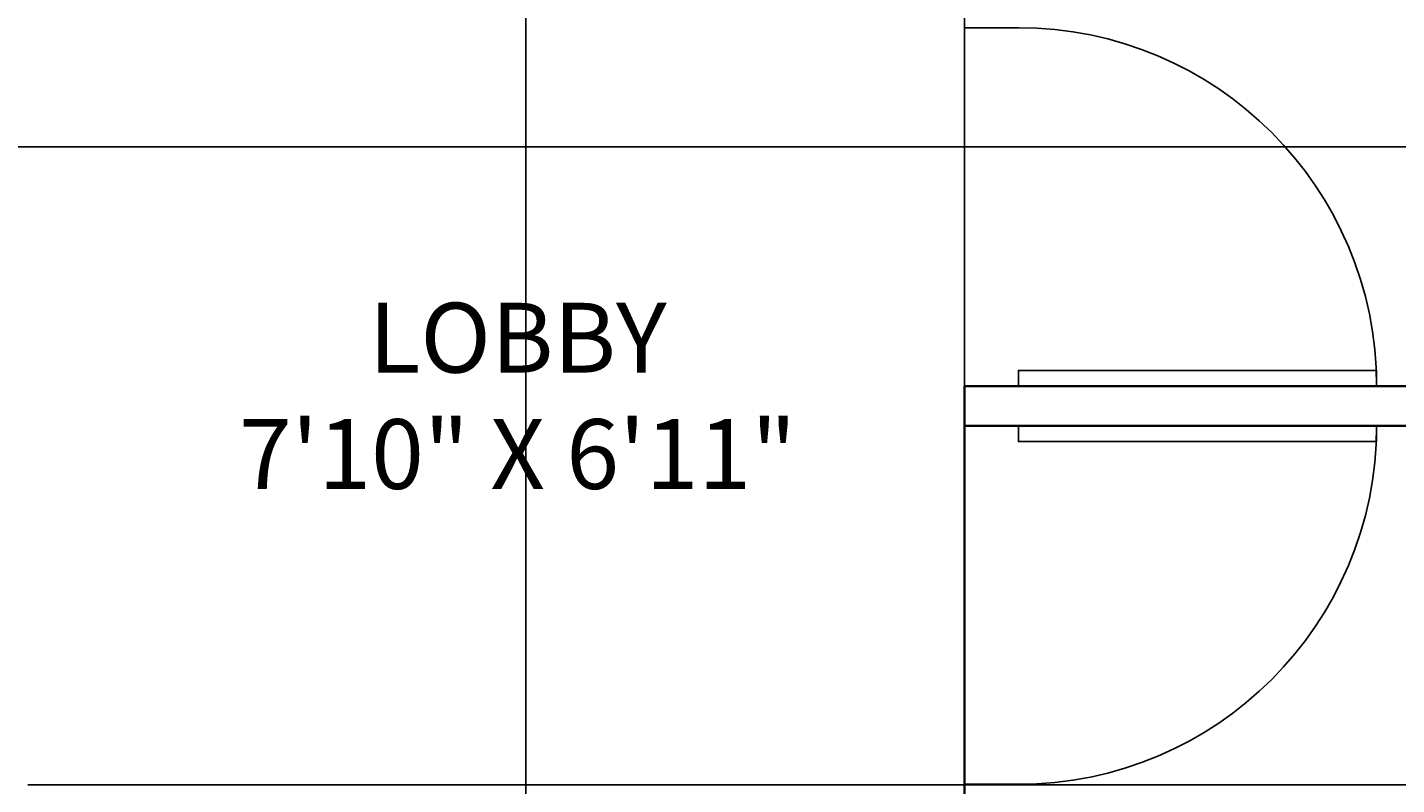
# Model space of a CAD drawing. Units: feet. Extents: x 105 to 1094, y -88 to 588.
# Tile 38 of 59: x 553 to 690, y 212 to 288. Entities that reach past the tile are written whole.
import ezdxf

# ---------------------------------------------------------------- set-up
doc = ezdxf.new("R2010")
doc.units = ezdxf.units.FT
doc.header["$MEASUREMENT"] = 0
for name, color, linetype, lineweight in [('A-ANNO-DIMS', 2, 'Continuous', 18), ('A-AREA-IDEN', 7, 'Continuous', 18), ('A-DOOR', 3, 'Continuous', 25), ('A-WALL', 7, 'Continuous', 35)]:
    doc.layers.add(name, color=color, linetype=linetype, lineweight=lineweight)
doc.styles.get("Standard").update_dxf_attribs({"font": 'arial.ttf'})
doc.dimstyles.get("Standard").update_dxf_attribs({"dimtxt": 0.18, "dimasz": 0.18, "dimexe": 0.18, "dimexo": 0.0625, "dimgap": 0.09, "dimtad": 0, "dimtih": 1, "dimtoh": 1, "dimdec": 4, "dimzin": 0, "dimdsep": 46, "dimtxsty": 'Standard', "dimcen": 0.09, "dimadec": 0, "dimazin": 0, "dimtfac": 1, "dimtdec": 4, "dimtofl": 0, "dimtmove": 0, "dimatfit": 3, "dimfxl": 1, "dimtolj": 1, "dimtzin": 0, "dimarcsym": 0})

# ---------------------------------------------------------------- blocks, each defined once
blk = doc.blocks.new('*U3')
for p, q in [((0, 0), (0, -6)), ((-40, 0), (-40, -6))]:
    blk.add_line(p, q)
blk.add_lwpolyline([(0, 0), (0, 40), (-1.75, 40), (-1.75, 0)], close=True)
blk.add_arc((0, 0), 40, 90, 180)
blk = doc.blocks.new('*D20')
at = {"layer": 'A-ANNO-DIMS', "color": 0, "lineweight": -2, "transparency": 16777216}
for p, q in [((150.69, 276.02), (150.69, -88.15)), ((1048.69, 276.02), (1048.69, -88.15)), ((150.87, -87.97), (599.4, -87.97)), ((1048.51, -87.97), (599.98, -87.97))]:
    blk.add_line(p, q, dxfattribs=at)
at = {"layer": 'A-ANNO-DIMS', "color": 0, "transparency": 16777216}
for points in [[(150.87, -87.94), (150.87, -88), (150.69, -87.97)], [(1048.51, -87.94), (1048.51, -88), (1048.69, -87.97)]]:
    blk.add_solid(points, dxfattribs=at)
at = {"layer": 'Defpoints', "color": 0, "transparency": 16777216}
for p in [(150.69, 276.08), (1048.69, 276.08), (1048.69, -87.97)]:
    blk.add_point(p, dxfattribs=at)
at = {"layer": 'A-ANNO-DIMS', "color": 0, "transparency": 16777216, "insert": (599.69, -87.97), "char_height": 0.18, "attachment_point": 5}
blk.add_mtext('\\A1;898', dxfattribs=at)
blk = doc.blocks.new('*D21')
at = {"layer": 'A-ANNO-DIMS', "color": 0, "lineweight": -2, "transparency": 16777216}
for p, q in [((849.63, 543.08), (105.46, 543.08)), ((105.64, 542.9), (105.64, 250.26)), ((105.64, -42.74), (105.64, 249.9)), ((849.63, -42.92), (105.46, -42.92))]:
    blk.add_line(p, q, dxfattribs=at)
at = {"layer": 'A-ANNO-DIMS', "color": 0, "transparency": 16777216}
for points in [[(105.61, 542.9), (105.67, 542.9), (105.64, 543.08)], [(105.61, -42.74), (105.67, -42.74), (105.64, -42.92)]]:
    blk.add_solid(points, dxfattribs=at)
at = {"layer": 'Defpoints', "color": 0, "transparency": 16777216}
for p in [(105.64, 543.08), (849.69, 543.08), (849.69, -42.92)]:
    blk.add_point(p, dxfattribs=at)
at = {"layer": 'A-ANNO-DIMS', "color": 0, "transparency": 16777216, "insert": (105.64, 250.08), "char_height": 0.18, "attachment_point": 5}
blk.add_mtext('\\A1;586', dxfattribs=at)
blk = doc.blocks.new('*D34')
at = {"layer": 'A-ANNO-DIMS', "color": 0, "lineweight": -2, "transparency": 16777216}
for p, q in [((552.75, 295.08), (1093.92, 295.08)), ((1093.74, 294.9), (1093.74, 253.76)), ((1093.74, 212.26), (1093.74, 253.4)), ((552.75, 212.08), (1093.92, 212.08))]:
    blk.add_line(p, q, dxfattribs=at)
at = {"layer": 'A-ANNO-DIMS', "color": 0, "transparency": 16777216}
for points in [[(1093.71, 294.9), (1093.77, 294.9), (1093.74, 295.08)], [(1093.71, 212.26), (1093.77, 212.26), (1093.74, 212.08)]]:
    blk.add_solid(points, dxfattribs=at)
at = {"layer": 'Defpoints', "color": 0, "transparency": 16777216}
for p in [(552.69, 295.08), (552.69, 212.08), (1093.74, 212.08)]:
    blk.add_point(p, dxfattribs=at)
at = {"layer": 'A-ANNO-DIMS', "color": 0, "transparency": 16777216, "insert": (1093.74, 253.58), "char_height": 0.18, "attachment_point": 5}
blk.add_mtext('\\A1;83', dxfattribs=at)
blk = doc.blocks.new('*D49')
at = {"layer": 'A-ANNO-DIMS', "color": 0, "lineweight": -2, "transparency": 16777216}
for p, q in [((602.69, 295.02), (602.69, -88.15)), ((646.69, 295.02), (646.69, -88.15)), ((602.87, -87.97), (624.47, -87.97)), ((646.51, -87.97), (624.91, -87.97))]:
    blk.add_line(p, q, dxfattribs=at)
at = {"layer": 'A-ANNO-DIMS', "color": 0, "transparency": 16777216}
for points in [[(602.87, -87.94), (602.87, -88), (602.69, -87.97)], [(646.51, -87.94), (646.51, -88), (646.69, -87.97)]]:
    blk.add_solid(points, dxfattribs=at)
at = {"layer": 'Defpoints', "color": 0, "transparency": 16777216}
for p in [(602.69, 295.08), (646.69, 295.08), (646.69, -87.97)]:
    blk.add_point(p, dxfattribs=at)
at = {"layer": 'A-ANNO-DIMS', "color": 0, "transparency": 16777216, "insert": (624.69, -87.97), "char_height": 0.18, "attachment_point": 5}
blk.add_mtext('\\A1;44', dxfattribs=at)
blk = doc.blocks.new('*D54')
at = {"layer": 'A-ANNO-DIMS', "color": 0, "lineweight": -2, "transparency": 16777216}
for p, q in [((294.75, 296.08), (1093.92, 296.08)), ((1093.74, 295.9), (1093.74, 286.26)), ((1093.74, 276.26), (1093.74, 285.9)), ((294.75, 276.08), (1093.92, 276.08))]:
    blk.add_line(p, q, dxfattribs=at)
at = {"layer": 'A-ANNO-DIMS', "color": 0, "transparency": 16777216}
for points in [[(1093.71, 295.9), (1093.77, 295.9), (1093.74, 296.08)], [(1093.71, 276.26), (1093.77, 276.26), (1093.74, 276.08)]]:
    blk.add_solid(points, dxfattribs=at)
at = {"layer": 'Defpoints', "color": 0, "transparency": 16777216}
for p in [(294.69, 296.08), (1093.74, 296.08), (294.69, 276.08)]:
    blk.add_point(p, dxfattribs=at)
at = {"layer": 'A-ANNO-DIMS', "color": 0, "transparency": 16777216, "insert": (1093.74, 286.08), "char_height": 0.18, "attachment_point": 5}
blk.add_mtext('\\A1;20', dxfattribs=at)

msp = doc.modelspace()

# ---------------------------------------------------------------- linework, layer by layer
at = {"layer": 'A-WALL'}
for p, q in [((646.6883, 252.0812), (772.6883, 252.0812)), ((646.6883, 252.0812), (646.6883, 248.0812)), ((646.6883, 252.0812), (828.6883, 252.0812)), ((646.6883, 248.0812), (646.6883, 252.0812)), ((646.6883, 248.0812), (828.6883, 248.0812)), ((646.6883, 248.0812), (646.6883, 140.0812)), ((646.6883, 248.0812), (772.6883, 248.0812))]:
    msp.add_line(p, q, dxfattribs=at)

# ---------------------------------------------------------------- block references
at = {"layer": 'A-DOOR', "yscale": 0.8984622266767051, "zscale": 0.8984622266767051, "rotation": 270}
for p, xscale in [((652.0791, 252.0812), 0.8984622266767051), ((652.0791, 248.0812), -0.8984622266767051)]:
    msp.add_blockref('*U3', p, dxfattribs=dict(at, xscale=xscale))

# ---------------------------------------------------------------- texts
at = {"layer": 'A-AREA-IDEN', "insert": (552.6883, 260.43), "char_height": 7, "attachment_point": 1}
msp.add_mtext_dynamic_manual_height_columns('\\pxqc;LOBBY \\P7\'10" X 6\'11"', width=98.34246, gutter_width=1, heights=[0], dxfattribs=at)

# ---------------------------------------------------------------- dimensions: what is measured, and where the dimension line sits
at = {"layer": 'A-ANNO-DIMS'}
for base, p1, p2, picture, middle in [((105.6383, 543.0812), (849.6883, -42.9188), (849.6883, 543.0812), '*D21', (105.6383, 250.0812)), ((1093.7383, 296.0812), (294.6883, 276.0812), (294.6883, 296.0812), '*D54', (1093.7383, 286.0812)), ((1093.7383, 212.0812), (552.6883, 295.0812), (552.6883, 212.0812), '*D34', (1093.7383, 253.5812))]:
    dim = msp.add_linear_dim(base=base, p1=p1, p2=p2, angle=90, dimstyle='Standard', override={"dimdec": 0, "dimlfac": 1, "dimrnd": 0, "dimzin": 0, "dimdsep": 46, "dimlunit": 2}, dxfattribs=at)
    dim.commit()
    dim.dimension.update_dxf_attribs({"geometry": picture, "text_midpoint": middle})
for base, p1, p2, picture, middle in [((646.6883, -87.9688), (602.6883, 295.0812), (646.6883, 295.0812), '*D49', (624.6883, -87.9688)), ((1048.6883, -87.9688), (150.6883, 276.0812), (1048.6883, 276.0812), '*D20', (599.6883, -87.9688))]:
    dim = msp.add_linear_dim(base=base, p1=p1, p2=p2, dimstyle='Standard', override={"dimdec": 0, "dimlfac": 1, "dimrnd": 0, "dimzin": 0, "dimdsep": 46, "dimlunit": 2}, dxfattribs=at)
    dim.commit()
    dim.dimension.update_dxf_attribs({"geometry": picture, "text_midpoint": middle})

doc.saveas('drawing.dxf')
